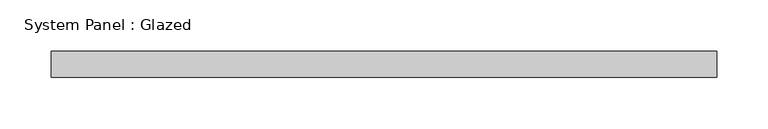
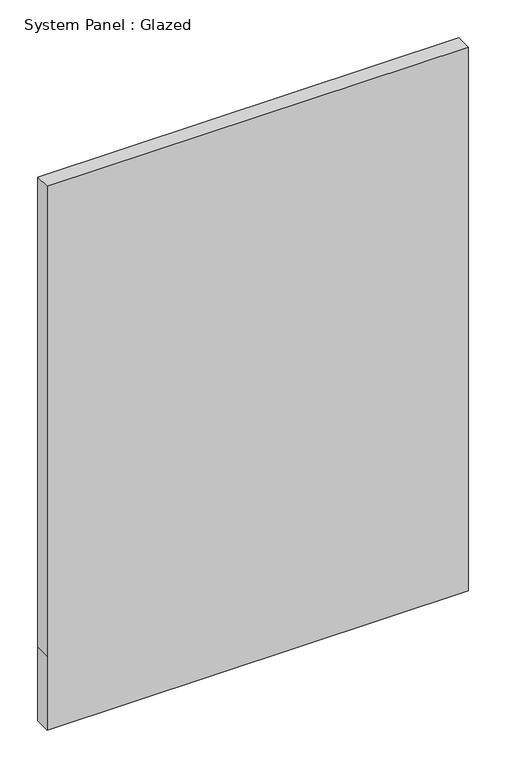
"""IFC4 building model written with IfcOpenShell, lengths in millimetres: plate geometry, System Panel : Glazed."""

from ifc_helpers import new_model, si_unit, frame, origin, place, context, project, spatial, polyline, outline, extrude, source, transform, mapped, element, save


def system_panel_glazed_8162a39b(model_context):
    return source(origin(), model_context, "Body", "SweptSolid", [
        extrude(outline(polyline([(0.0, -323.85), (0.0, 323.85), (120.65, 323.85), (884.4809713, 323.85), (884.4809713, -323.85), (120.65, -323.85), (0.0, -323.85)])), frame((0.0, 19.05, 0.0), z_axis=(0.0, 1.0, 0.0), x_axis=(0.0, 0.0, 1.0)), (0.0, 0.0, 1.0), 25.4),
    ])


if __name__ == "__main__":
    model = new_model("IFC4")
    model_context = context("Model", 3, world=origin())
    ifc_project = project(units=[si_unit("LENGTHUNIT", "METRE", prefix="MILLI")], contexts=[model_context])
    site = spatial("IfcSite", under=ifc_project)
    building = spatial("IfcBuilding", under=site)
    placement = place(None, origin())
    system_panel_glazed_shape = system_panel_glazed_8162a39b(model_context)
    element("IfcPlate", 1, ObjectType="System Panel : Glazed", at=placement, inside=building, context=model_context, shape_type="MappedRepresentation", body=[
        mapped(system_panel_glazed_shape, transform((0.0, 0.0, 0.0), x_axis=(1.0, 0.0, 0.0), y_axis=(0.0, 1.0, 0.0), z_axis=(0.0, 0.0, 1.0))),
    ])
    save(model, "model.ifc")

# Revit data of these elements
# Type "System Panel : Glazed"
#   Construction Type Id = "GSP4R"
#   Analytic Construction = "1/8 in Pilkington single glazing"
#   Visual Light Transmittance = 0.9
#   Solar Heat Gain Coefficient = 0.86
#   Heat Transfer Coefficient (U) = 1.18115 BTU/(h·ft²·°F)
#   Define Thermal Properties by = 1
# Element 1 (IfcPlate, "System Panel : Glazed")
#   Materials on its faces: "Glass"
# Materials
#   "Glass": class "Glass", colour RGB 0 128 192, transparency 0.75, Description = "Soda Lime Glass", Cost = 0
